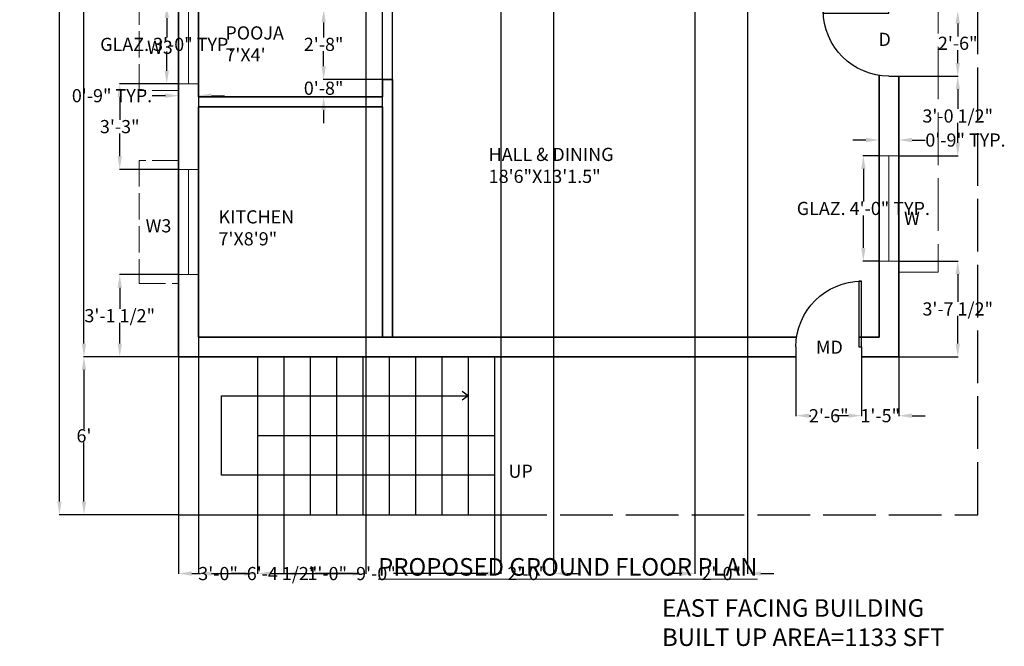
# Model space of a CAD drawing. Units: inches. Extents: x 515 to 964, y 435 to 999.
# Tile 1 of 2: x 515 to 964, y 435 to 721. Entities that reach past the tile are written whole.
import ezdxf

# ---------------------------------------------------------------- set-up
doc = ezdxf.new("R2010")
doc.units = ezdxf.units.IN
doc.header["$MEASUREMENT"] = 0
doc.linetypes.add('ACAD_ISO02W100', pattern=[15, 12, -3])
for name, color, linetype, lineweight in [('A-ANNO-DIMS', 2, 'Continuous', 18), ('A-ANNO-TEXT', 7, 'Continuous', 18), ('A-AREA-IDEN', 7, 'Continuous', 18), ('A-DOOR', 3, 'Continuous', 25), ('A-FLOR-OVHD', 8, 'ACAD_ISO02W100', 18), ('A-FLOR-STRS', 7, 'Continuous', 25), ('A-GLAZ', 4, 'Continuous', 18), ('A-WALL', 7, 'Continuous', 35), ('C-PROP', 8, 'ACAD_ISO02W100', 25)]:
    doc.layers.add(name, color=color, linetype=linetype, lineweight=lineweight)
doc.styles.get("Standard").update_dxf_attribs({"font": 'arial.ttf'})
doc.dimstyles.get("Standard").update_dxf_attribs({"dimtxt": 6, "dimasz": 6, "dimexe": 0.18, "dimexo": 0.0625, "dimgap": 0.09, "dimtad": 0, "dimtih": 1, "dimtoh": 1, "dimdec": 0, "dimzin": 0, "dimdsep": 46, "dimlunit": 3, "dimtxsty": 'Standard', "dimcen": 0.09, "dimadec": 0, "dimazin": 0, "dimtfac": 1, "dimtdec": 0, "dimtofl": 0, "dimtmove": 0, "dimatfit": 3, "dimfxl": 1, "dimtolj": 1, "dimtzin": 0, "dimarcsym": 0})

# ---------------------------------------------------------------- blocks, each defined once
blk = doc.blocks.new('*U2')
for p, q in [((0, 0), (0, -6)), ((40, 0), (40, -6))]:
    blk.add_line(p, q)
blk.add_lwpolyline([(0, 0), (0, 40), (1.75, 40), (1.75, 0)], close=True)
blk.add_arc((0, 0), 40, 0, 90)
blk = doc.blocks.new('*D5')
at = {"layer": 'A-ANNO-DIMS', "color": 0, "lineweight": -2, "transparency": 16777216}
for p, q in [((587.7, 945.51), (544.42, 945.51)), ((544.6, 939.51), (544.6, 759.42)), ((544.6, 573.01), (544.6, 753.11)), ((587.7, 567.01), (544.42, 567.01))]:
    blk.add_line(p, q, dxfattribs=at)
at = {"layer": 'A-ANNO-DIMS', "color": 0, "transparency": 16777216}
for points in [[(543.6, 939.51), (545.6, 939.51), (544.6, 945.51)], [(543.6, 573.01), (545.6, 573.01), (544.6, 567.01)]]:
    blk.add_solid(points, dxfattribs=at)
at = {"layer": 'Defpoints', "color": 0, "transparency": 16777216}
for p in [(587.76, 945.51), (544.6, 567.01), (587.76, 567.01)]:
    blk.add_point(p, dxfattribs=at)
at = {"layer": 'A-ANNO-DIMS', "color": 0, "transparency": 16777216, "insert": (544.6, 756.26), "char_height": 6, "attachment_point": 5}
blk.add_mtext('\\A1;31\'-7"', dxfattribs=at)
blk = doc.blocks.new('*D6')
at = {"layer": 'A-ANNO-DIMS', "color": 0, "lineweight": -2, "transparency": 16777216}
for p, q in [((587.7, 567.01), (544.42, 567.01)), ((544.6, 561.01), (544.6, 534.16)), ((544.6, 501.01), (544.6, 527.86)), ((587.7, 495.01), (544.42, 495.01))]:
    blk.add_line(p, q, dxfattribs=at)
at = {"layer": 'A-ANNO-DIMS', "color": 0, "transparency": 16777216}
for points in [[(543.6, 561.01), (545.6, 561.01), (544.6, 567.01)], [(543.6, 501.01), (545.6, 501.01), (544.6, 495.01)]]:
    blk.add_solid(points, dxfattribs=at)
at = {"layer": 'Defpoints', "color": 0, "transparency": 16777216}
for p in [(587.76, 567.01), (544.6, 495.01), (587.76, 495.01)]:
    blk.add_point(p, dxfattribs=at)
at = {"layer": 'A-ANNO-DIMS', "color": 0, "transparency": 16777216, "insert": (544.6, 531.01), "char_height": 6, "attachment_point": 5}
blk.add_mtext("\\A1;6'", dxfattribs=at)
blk = doc.blocks.new('GLAZ-48IN')
blk.add_line((4.5, 0), (4.5, 48))
blk.add_lwpolyline([(0, 0), (0, 48), (9, 48), (9, 0)], close=True)
blk = doc.blocks.new('GLAZ-36IN')
blk.add_line((0, 4.5), (36, 4.5))
blk.add_lwpolyline([(0, 9), (36, 9), (36, 0), (0, 0)], close=True)
blk = doc.blocks.new('*D10')
at = {"layer": 'A-ANNO-DIMS', "color": 0, "lineweight": -2, "transparency": 16777216}
for p, q in [((907.2, 658.68), (899.88, 658.68)), ((900.06, 652.68), (900.06, 637.87)), ((900.06, 616.68), (900.06, 631.49)), ((907.2, 610.68), (899.88, 610.68))]:
    blk.add_line(p, q, dxfattribs=at)
at = {"layer": 'A-ANNO-DIMS', "color": 0, "transparency": 16777216}
for points in [[(899.06, 652.68), (901.06, 652.68), (900.06, 658.68)], [(899.06, 616.68), (901.06, 616.68), (900.06, 610.68)]]:
    blk.add_solid(points, dxfattribs=at)
at = {"layer": 'Defpoints', "color": 0, "transparency": 16777216}
for p in [(900.06, 658.68), (907.26, 658.68), (907.26, 610.68)]:
    blk.add_point(p, dxfattribs=at)
at = {"layer": 'A-ANNO-DIMS', "color": 0, "transparency": 16777216, "insert": (900.06, 634.68), "char_height": 6, "attachment_point": 5}
blk.add_mtext('\\A1;GLAZ. 4\'-0" TYP.', dxfattribs=at)
blk = doc.blocks.new('*D11')
at = {"layer": 'A-ANNO-DIMS', "color": 0, "lineweight": -2, "transparency": 16777216}
for p, q in [((901.26, 665.88), (895.26, 665.88)), ((907.26, 658.74), (907.26, 666.06)), ((916.26, 658.74), (916.26, 666.06)), ((922.26, 665.88), (928.26, 665.88))]:
    blk.add_line(p, q, dxfattribs=at)
at = {"layer": 'A-ANNO-DIMS', "color": 0, "transparency": 16777216}
for points in [[(901.26, 666.88), (901.26, 664.88), (907.26, 665.88)], [(922.26, 666.88), (922.26, 664.88), (916.26, 665.88)]]:
    blk.add_solid(points, dxfattribs=at)
at = {"layer": 'Defpoints', "color": 0, "transparency": 16777216}
for p in [(916.26, 665.88), (907.26, 658.68), (916.26, 658.68)]:
    blk.add_point(p, dxfattribs=at)
at = {"layer": 'A-ANNO-DIMS', "color": 0, "transparency": 16777216, "insert": (946.64, 665.88), "char_height": 6, "attachment_point": 5}
blk.add_mtext('\\A1;0\'-9" TYP.', dxfattribs=at)
blk = doc.blocks.new('*D12')
at = {"layer": 'A-ANNO-DIMS', "color": 0, "lineweight": -2, "transparency": 16777216}
for p, q in [((587.7, 727.51), (582.18, 727.51)), ((582.36, 721.51), (582.36, 712.71)), ((582.36, 697.51), (582.36, 706.32)), ((587.7, 691.51), (582.18, 691.51))]:
    blk.add_line(p, q, dxfattribs=at)
at = {"layer": 'A-ANNO-DIMS', "color": 0, "transparency": 16777216}
for points in [[(581.36, 721.51), (583.36, 721.51), (582.36, 727.51)], [(581.36, 697.51), (583.36, 697.51), (582.36, 691.51)]]:
    blk.add_solid(points, dxfattribs=at)
at = {"layer": 'Defpoints', "color": 0, "transparency": 16777216}
for p in [(582.36, 727.51), (587.76, 727.51), (587.76, 691.51)]:
    blk.add_point(p, dxfattribs=at)
at = {"layer": 'A-ANNO-DIMS', "color": 0, "transparency": 16777216, "insert": (582.36, 709.51), "char_height": 6, "attachment_point": 5}
blk.add_mtext('\\A1;GLAZ. 3\'-0" TYP.', dxfattribs=at)
blk = doc.blocks.new('*D13')
at = {"layer": 'A-ANNO-DIMS', "color": 0, "lineweight": -2, "transparency": 16777216}
for p, q in [((587.76, 691.45), (587.76, 685.93)), ((596.76, 691.45), (596.76, 685.93)), ((581.76, 686.11), (575.76, 686.11)), ((602.76, 686.11), (608.76, 686.11))]:
    blk.add_line(p, q, dxfattribs=at)
at = {"layer": 'A-ANNO-DIMS', "color": 0, "transparency": 16777216}
for points in [[(581.76, 687.11), (581.76, 685.11), (587.76, 686.11)], [(602.76, 687.11), (602.76, 685.11), (596.76, 686.11)]]:
    blk.add_solid(points, dxfattribs=at)
at = {"layer": 'Defpoints', "color": 0, "transparency": 16777216}
for p in [(587.76, 691.51), (596.76, 691.51), (587.76, 686.11)]:
    blk.add_point(p, dxfattribs=at)
at = {"layer": 'A-ANNO-DIMS', "color": 0, "transparency": 16777216, "insert": (557.38, 686.11), "char_height": 6, "attachment_point": 5}
blk.add_mtext('\\A1;0\'-9" TYP.', dxfattribs=at)
blk = doc.blocks.new('*D17')
at = {"layer": 'A-ANNO-DIMS', "color": 0, "lineweight": -2, "transparency": 16777216}
for p, q in [((667.63, 963.51), (533.24, 963.51)), ((533.42, 957.51), (533.42, 732.46)), ((533.42, 501.01), (533.42, 726.07)), ((587.7, 495.01), (533.24, 495.01))]:
    blk.add_line(p, q, dxfattribs=at)
at = {"layer": 'A-ANNO-DIMS', "color": 0, "transparency": 16777216}
for points in [[(532.42, 957.51), (534.42, 957.51), (533.42, 963.51)], [(532.42, 501.01), (534.42, 501.01), (533.42, 495.01)]]:
    blk.add_solid(points, dxfattribs=at)
at = {"layer": 'Defpoints', "color": 0, "transparency": 16777216}
for p in [(533.42, 963.51), (667.69, 963.51), (587.76, 495.01)]:
    blk.add_point(p, dxfattribs=at)
at = {"layer": 'A-ANNO-DIMS', "color": 0, "transparency": 16777216, "insert": (533.42, 729.26), "char_height": 6, "attachment_point": 5}
blk.add_mtext('\\A1;39\'-0 1/2"', dxfattribs=at)
blk = doc.blocks.new('*D18')
at = {"layer": 'A-ANNO-DIMS', "color": 0, "lineweight": -2, "transparency": 16777216}
for p, q in [((623.76, 494.95), (623.76, 467.98)), ((731.76, 494.95), (731.76, 467.98)), ((629.76, 468.16), (669.7, 468.16)), ((725.76, 468.16), (685.83, 468.16))]:
    blk.add_line(p, q, dxfattribs=at)
at = {"layer": 'A-ANNO-DIMS', "color": 0, "transparency": 16777216}
for points in [[(629.76, 469.16), (629.76, 467.16), (623.76, 468.16)], [(725.76, 469.16), (725.76, 467.16), (731.76, 468.16)]]:
    blk.add_solid(points, dxfattribs=at)
at = {"layer": 'Defpoints', "color": 0, "transparency": 16777216}
for p in [(623.76, 495.01), (731.76, 495.01), (731.76, 468.16)]:
    blk.add_point(p, dxfattribs=at)
at = {"layer": 'A-ANNO-DIMS', "color": 0, "transparency": 16777216, "insert": (677.76, 468.16), "char_height": 6, "attachment_point": 5}
blk.add_mtext('\\A1;9\'-0"', dxfattribs=at)
blk = doc.blocks.new('*D19')
at = {"layer": 'A-ANNO-DIMS', "color": 0, "lineweight": -2, "transparency": 16777216}
for p, q in [((587.76, 494.95), (587.76, 467.98)), ((623.76, 494.95), (623.76, 467.98)), ((593.76, 468.16), (597.7, 468.16)), ((617.76, 468.16), (613.82, 468.16))]:
    blk.add_line(p, q, dxfattribs=at)
at = {"layer": 'A-ANNO-DIMS', "color": 0, "transparency": 16777216}
for points in [[(593.76, 469.16), (593.76, 467.16), (587.76, 468.16)], [(617.76, 469.16), (617.76, 467.16), (623.76, 468.16)]]:
    blk.add_solid(points, dxfattribs=at)
at = {"layer": 'Defpoints', "color": 0, "transparency": 16777216}
for p in [(587.76, 495.01), (623.76, 495.01), (623.76, 468.16)]:
    blk.add_point(p, dxfattribs=at)
at = {"layer": 'A-ANNO-DIMS', "color": 0, "transparency": 16777216, "insert": (605.76, 468.16), "char_height": 6, "attachment_point": 5}
blk.add_mtext('\\A1;3\'-0"', dxfattribs=at)
blk = doc.blocks.new('*D20')
at = {"layer": 'A-ANNO-DIMS', "color": 0, "lineweight": -2, "transparency": 16777216}
for p, q in [((623.76, 494.95), (623.76, 467.98)), ((635.76, 494.95), (635.76, 467.98)), ((617.76, 468.16), (611.76, 468.16)), ((641.76, 468.16), (647.76, 468.16))]:
    blk.add_line(p, q, dxfattribs=at)
at = {"layer": 'A-ANNO-DIMS', "color": 0, "transparency": 16777216}
for points in [[(617.76, 469.16), (617.76, 467.16), (623.76, 468.16)], [(641.76, 469.16), (641.76, 467.16), (635.76, 468.16)]]:
    blk.add_solid(points, dxfattribs=at)
at = {"layer": 'Defpoints', "color": 0, "transparency": 16777216}
for p in [(623.76, 495.01), (635.76, 495.01), (635.76, 468.16)]:
    blk.add_point(p, dxfattribs=at)
at = {"layer": 'A-ANNO-DIMS', "color": 0, "transparency": 16777216, "insert": (655.54, 468.16), "char_height": 6, "attachment_point": 5}
blk.add_mtext('\\A1;1\'-0"', dxfattribs=at)
blk = doc.blocks.new('*D21')
at = {"layer": 'A-ANNO-DIMS', "color": 0, "lineweight": -2, "transparency": 16777216}
for p, q in [((869.29, 566.95), (869.29, 539.98)), ((899.29, 566.95), (899.29, 539.98)), ((875.29, 540.16), (876.17, 540.16)), ((893.29, 540.16), (892.4, 540.16))]:
    blk.add_line(p, q, dxfattribs=at)
at = {"layer": 'A-ANNO-DIMS', "color": 0, "transparency": 16777216}
for points in [[(875.29, 541.16), (875.29, 539.16), (869.29, 540.16)], [(893.29, 541.16), (893.29, 539.16), (899.29, 540.16)]]:
    blk.add_solid(points, dxfattribs=at)
at = {"layer": 'Defpoints', "color": 0, "transparency": 16777216}
for p in [(869.29, 567.01), (899.29, 567.01), (869.29, 540.16)]:
    blk.add_point(p, dxfattribs=at)
at = {"layer": 'A-ANNO-DIMS', "color": 0, "transparency": 16777216, "insert": (884.29, 540.16), "char_height": 6, "attachment_point": 5}
blk.add_mtext('\\A1;2\'-6"', dxfattribs=at)
blk = doc.blocks.new('*D22')
at = {"layer": 'A-ANNO-DIMS', "color": 0, "lineweight": -2, "transparency": 16777216}
for p, q in [((899.29, 566.95), (899.29, 539.98)), ((916.26, 566.95), (916.26, 539.98)), ((893.29, 540.16), (887.29, 540.16)), ((922.26, 540.16), (928.26, 540.16))]:
    blk.add_line(p, q, dxfattribs=at)
at = {"layer": 'A-ANNO-DIMS', "color": 0, "transparency": 16777216}
for points in [[(893.29, 541.16), (893.29, 539.16), (899.29, 540.16)], [(922.26, 541.16), (922.26, 539.16), (916.26, 540.16)]]:
    blk.add_solid(points, dxfattribs=at)
at = {"layer": 'Defpoints', "color": 0, "transparency": 16777216}
for p in [(899.29, 567.01), (916.26, 567.01), (899.29, 540.16)]:
    blk.add_point(p, dxfattribs=at)
at = {"layer": 'A-ANNO-DIMS', "color": 0, "transparency": 16777216, "insert": (907.77, 540.16), "char_height": 6, "attachment_point": 5}
blk.add_mtext('\\A1;1\'-5"', dxfattribs=at)
blk = doc.blocks.new('*D23')
at = {"layer": 'A-ANNO-DIMS', "color": 0, "lineweight": -2, "transparency": 16777216}
for p, q in [((674.76, 990.36), (668.76, 990.36)), ((680.76, 576.07), (680.76, 990.54)), ((685.26, 576.07), (685.26, 990.54)), ((691.26, 990.36), (697.26, 990.36))]:
    blk.add_line(p, q, dxfattribs=at)
at = {"layer": 'A-ANNO-DIMS', "color": 0, "transparency": 16777216}
for points in [[(674.76, 991.36), (674.76, 989.36), (680.76, 990.36)], [(691.26, 991.36), (691.26, 989.36), (685.26, 990.36)]]:
    blk.add_solid(points, dxfattribs=at)
at = {"layer": 'Defpoints', "color": 0, "transparency": 16777216}
for p in [(685.26, 990.36), (680.76, 576.01), (685.26, 576.01)]:
    blk.add_point(p, dxfattribs=at)
at = {"layer": 'A-ANNO-DIMS', "color": 0, "transparency": 16777216, "insert": (712.32, 990.36), "char_height": 6, "attachment_point": 5}
blk.add_mtext('\\A1;0\'-4 1/2"', dxfattribs=at)
blk = doc.blocks.new('*D24')
at = {"layer": 'A-ANNO-DIMS', "color": 0, "lineweight": -2, "transparency": 16777216}
for p, q in [((596.76, 936.45), (596.76, 467.98)), ((673.1, 936.45), (673.1, 467.98)), ((602.76, 468.16), (619.86, 468.16)), ((667.1, 468.16), (650, 468.16))]:
    blk.add_line(p, q, dxfattribs=at)
at = {"layer": 'A-ANNO-DIMS', "color": 0, "transparency": 16777216}
for points in [[(602.76, 469.16), (602.76, 467.16), (596.76, 468.16)], [(667.1, 469.16), (667.1, 467.16), (673.1, 468.16)]]:
    blk.add_solid(points, dxfattribs=at)
at = {"layer": 'Defpoints', "color": 0, "transparency": 16777216}
for p in [(596.76, 936.51), (673.1, 936.51), (673.1, 468.16)]:
    blk.add_point(p, dxfattribs=at)
at = {"layer": 'A-ANNO-DIMS', "color": 0, "transparency": 16777216, "insert": (634.93, 468.16), "char_height": 6, "attachment_point": 5}
blk.add_mtext('\\A1;6\'-4 1/2"', dxfattribs=at)
blk = doc.blocks.new('*D25')
at = {"layer": 'A-ANNO-DIMS', "color": 0, "lineweight": -2, "transparency": 16777216}
for p, q in [((734.760949, 936.449016), (734.760949, 467.981516)), ((758.760949, 936.449016), (758.760949, 467.981516)), ((728.760949, 468.161516), (722.760949, 468.161516)), ((764.760949, 468.161516), (770.760949, 468.161516))]:
    blk.add_line(p, q, dxfattribs=at)
at = {"layer": 'A-ANNO-DIMS', "color": 0, "transparency": 16777216}
for points in [[(728.760949, 469.161516), (728.760949, 467.161516), (734.760949, 468.161516)], [(764.760949, 469.161516), (764.760949, 467.161516), (758.760949, 468.161516)]]:
    blk.add_solid(points, dxfattribs=at)
at = {"layer": 'Defpoints', "color": 0, "transparency": 16777216}
for p in [(734.760949, 936.511516), (758.760949, 936.511516), (758.760949, 468.161516)]:
    blk.add_point(p, dxfattribs=at)
at = {"layer": 'A-ANNO-DIMS', "color": 0, "transparency": 16777216, "insert": (746.760949, 468.161516), "char_height": 6, "attachment_point": 5}
blk.add_mtext('\\A1;2\'-0"', dxfattribs=at)
blk = doc.blocks.new('*D26')
at = {"layer": 'A-ANNO-DIMS', "color": 0, "lineweight": -2, "transparency": 16777216}
for p, q in [((823.260949, 936.449016), (823.260949, 467.981516)), ((847.260949, 936.449016), (847.260949, 467.981516)), ((817.260949, 468.161516), (811.260949, 468.161516)), ((853.260949, 468.161516), (859.260949, 468.161516))]:
    blk.add_line(p, q, dxfattribs=at)
at = {"layer": 'A-ANNO-DIMS', "color": 0, "transparency": 16777216}
for points in [[(817.260949, 469.161516), (817.260949, 467.161516), (823.260949, 468.161516)], [(853.260949, 469.161516), (853.260949, 467.161516), (847.260949, 468.161516)]]:
    blk.add_solid(points, dxfattribs=at)
at = {"layer": 'Defpoints', "color": 0, "transparency": 16777216}
for p in [(823.260949, 936.511516), (847.260949, 936.511516), (847.260949, 468.161516)]:
    blk.add_point(p, dxfattribs=at)
at = {"layer": 'A-ANNO-DIMS', "color": 0, "transparency": 16777216, "insert": (835.260949, 468.161516), "char_height": 6, "attachment_point": 5}
blk.add_mtext('\\A1;2\'-0"', dxfattribs=at)
blk = doc.blocks.new('*D27')
at = {"layer": 'A-ANNO-DIMS', "color": 0, "lineweight": -2, "transparency": 16777216}
for p, q in [((587.7, 604.51), (560.73, 604.51)), ((560.91, 598.51), (560.91, 588.96)), ((560.91, 573.01), (560.91, 582.57)), ((587.7, 567.01), (560.73, 567.01))]:
    blk.add_line(p, q, dxfattribs=at)
at = {"layer": 'A-ANNO-DIMS', "color": 0, "transparency": 16777216}
for points in [[(559.91, 598.51), (561.91, 598.51), (560.91, 604.51)], [(559.91, 573.01), (561.91, 573.01), (560.91, 567.01)]]:
    blk.add_solid(points, dxfattribs=at)
at = {"layer": 'Defpoints', "color": 0, "transparency": 16777216}
for p in [(560.91, 604.51), (587.76, 604.51), (587.76, 567.01)]:
    blk.add_point(p, dxfattribs=at)
at = {"layer": 'A-ANNO-DIMS', "color": 0, "transparency": 16777216, "insert": (560.91, 585.76), "char_height": 6, "attachment_point": 5}
blk.add_mtext('\\A1;3\'-1 1/2"', dxfattribs=at)
blk = doc.blocks.new('*D28')
at = {"layer": 'A-ANNO-DIMS', "color": 0, "lineweight": -2, "transparency": 16777216}
for p, q in [((587.7, 691.51), (560.73, 691.51)), ((560.91, 685.51), (560.91, 675.17)), ((560.91, 658.51), (560.91, 668.86)), ((587.7, 652.51), (560.73, 652.51))]:
    blk.add_line(p, q, dxfattribs=at)
at = {"layer": 'A-ANNO-DIMS', "color": 0, "transparency": 16777216}
for points in [[(559.91, 685.51), (561.91, 685.51), (560.91, 691.51)], [(559.91, 658.51), (561.91, 658.51), (560.91, 652.51)]]:
    blk.add_solid(points, dxfattribs=at)
at = {"layer": 'Defpoints', "color": 0, "transparency": 16777216}
for p in [(560.91, 691.51), (587.76, 691.51), (587.76, 652.51)]:
    blk.add_point(p, dxfattribs=at)
at = {"layer": 'A-ANNO-DIMS', "color": 0, "transparency": 16777216, "insert": (560.91, 672.01), "char_height": 6, "attachment_point": 5}
blk.add_mtext('\\A1;3\'-3"', dxfattribs=at)
blk = doc.blocks.new('*D30')
at = {"layer": 'A-ANNO-DIMS', "color": 0, "lineweight": -2, "transparency": 16777216}
for p, q in [((916.32, 610.68), (943.29, 610.68)), ((943.11, 604.68), (943.11, 592.04)), ((943.11, 573.01), (943.11, 585.65)), ((916.32, 567.01), (943.29, 567.01))]:
    blk.add_line(p, q, dxfattribs=at)
at = {"layer": 'A-ANNO-DIMS', "color": 0, "transparency": 16777216}
for points in [[(942.11, 604.68), (944.11, 604.68), (943.11, 610.68)], [(942.11, 573.01), (944.11, 573.01), (943.11, 567.01)]]:
    blk.add_solid(points, dxfattribs=at)
at = {"layer": 'Defpoints', "color": 0, "transparency": 16777216}
for p in [(916.26, 610.68), (916.26, 567.01), (943.11, 567.01)]:
    blk.add_point(p, dxfattribs=at)
at = {"layer": 'A-ANNO-DIMS', "color": 0, "transparency": 16777216, "insert": (943.11, 588.85), "char_height": 6, "attachment_point": 5}
blk.add_mtext('\\A1;3\'-7 1/2"', dxfattribs=at)
blk = doc.blocks.new('*D31')
at = {"layer": 'A-ANNO-DIMS', "color": 0, "lineweight": -2, "transparency": 16777216}
for p, q in [((916.32, 695.01), (943.29, 695.01)), ((943.11, 689.01), (943.11, 680.04)), ((943.11, 664.68), (943.11, 673.65)), ((916.32, 658.68), (943.29, 658.68))]:
    blk.add_line(p, q, dxfattribs=at)
at = {"layer": 'A-ANNO-DIMS', "color": 0, "transparency": 16777216}
for points in [[(942.11, 689.01), (944.11, 689.01), (943.11, 695.01)], [(942.11, 664.68), (944.11, 664.68), (943.11, 658.68)]]:
    blk.add_solid(points, dxfattribs=at)
at = {"layer": 'Defpoints', "color": 0, "transparency": 16777216}
for p in [(916.26, 695.01), (916.26, 658.68), (943.11, 658.68)]:
    blk.add_point(p, dxfattribs=at)
at = {"layer": 'A-ANNO-DIMS', "color": 0, "transparency": 16777216, "insert": (943.11, 676.85), "char_height": 6, "attachment_point": 5}
blk.add_mtext('\\A1;3\'-0 1/2"', dxfattribs=at)
blk = doc.blocks.new('*D32')
at = {"layer": 'A-ANNO-DIMS', "color": 0, "lineweight": -2, "transparency": 16777216}
for p, q in [((916.32, 725.01), (943.29, 725.01)), ((943.11, 719.01), (943.11, 713.16)), ((943.11, 701.01), (943.11, 706.86)), ((916.32, 695.01), (943.29, 695.01))]:
    blk.add_line(p, q, dxfattribs=at)
at = {"layer": 'A-ANNO-DIMS', "color": 0, "transparency": 16777216}
for points in [[(942.11, 719.01), (944.11, 719.01), (943.11, 725.01)], [(942.11, 701.01), (944.11, 701.01), (943.11, 695.01)]]:
    blk.add_solid(points, dxfattribs=at)
at = {"layer": 'Defpoints', "color": 0, "transparency": 16777216}
for p in [(916.26, 725.01), (916.26, 695.01), (943.11, 695.01)]:
    blk.add_point(p, dxfattribs=at)
at = {"layer": 'A-ANNO-DIMS', "color": 0, "transparency": 16777216, "insert": (943.11, 710.01), "char_height": 6, "attachment_point": 5}
blk.add_mtext('\\A1;2\'-6"', dxfattribs=at)
blk = doc.blocks.new('*D34')
at = {"layer": 'A-ANNO-DIMS', "color": 0, "lineweight": -2, "transparency": 16777216}
for p, q in [((680.7, 725.51), (653.73, 725.51)), ((653.91, 719.51), (653.91, 712.66)), ((653.91, 699.51), (653.91, 706.36)), ((680.7, 693.51), (653.73, 693.51))]:
    blk.add_line(p, q, dxfattribs=at)
at = {"layer": 'A-ANNO-DIMS', "color": 0, "transparency": 16777216}
for points in [[(652.91, 719.51), (654.91, 719.51), (653.91, 725.51)], [(652.91, 699.51), (654.91, 699.51), (653.91, 693.51)]]:
    blk.add_solid(points, dxfattribs=at)
at = {"layer": 'Defpoints', "color": 0, "transparency": 16777216}
for p in [(653.91, 725.51), (680.76, 725.51), (680.76, 693.51)]:
    blk.add_point(p, dxfattribs=at)
at = {"layer": 'A-ANNO-DIMS', "color": 0, "transparency": 16777216, "insert": (653.91, 709.51), "char_height": 6, "attachment_point": 5}
blk.add_mtext('\\A1;2\'-8"', dxfattribs=at)
blk = doc.blocks.new('*D35')
at = {"layer": 'A-ANNO-DIMS', "color": 0, "lineweight": -2, "transparency": 16777216}
for p, q in [((653.910949, 699.511516), (653.910949, 705.511516)), ((680.698449, 693.511516), (653.730949, 693.511516)), ((680.698449, 685.511516), (653.730949, 685.511516)), ((653.910949, 679.511516), (653.910949, 673.511516))]:
    blk.add_line(p, q, dxfattribs=at)
at = {"layer": 'A-ANNO-DIMS', "color": 0, "transparency": 16777216}
for points in [[(652.910949, 699.511516), (654.910949, 699.511516), (653.910949, 693.511516)], [(652.910949, 679.511516), (654.910949, 679.511516), (653.910949, 685.511516)]]:
    blk.add_solid(points, dxfattribs=at)
at = {"layer": 'Defpoints', "color": 0, "transparency": 16777216}
for p in [(653.910949, 693.511516), (680.760949, 693.511516), (680.760949, 685.511516)]:
    blk.add_point(p, dxfattribs=at)
at = {"layer": 'A-ANNO-DIMS', "color": 0, "transparency": 16777216, "insert": (653.910949, 689.511516), "char_height": 6, "attachment_point": 5}
blk.add_mtext('\\A1;0\'-8"', dxfattribs=at)

msp = doc.modelspace()

# ---------------------------------------------------------------- linework, layer by layer
at = {"layer": 'A-FLOR-OVHD'}
for p, q in [((587.76, 656.62), (569.76, 656.62)), ((569.76, 656.62), (569.76, 600.39)), ((569.76, 600.39), (587.76, 600.39))]:
    msp.add_line(p, q, dxfattribs=at)
at = {"layer": 'A-FLOR-OVHD', "ltscale": 2}
msp.add_lwpolyline([(916.26, 828.46), (934.26, 828.46), (934.26, 605.63), (916.26, 605.63)], dxfattribs=at)
at = {"layer": 'A-FLOR-OVHD'}
msp.add_lwpolyline([(587.76, 688.47), (569.76, 688.47), (569.76, 731.11)], dxfattribs=at)
at = {"layer": 'A-FLOR-STRS'}
for p, q in [((587.76, 567.01), (587.76, 495.01)), ((623.76, 567.01), (623.76, 495.01)), ((635.76, 567.01), (635.76, 495.01)), ((647.76, 567.01), (647.76, 495.01)), ((659.76, 567.01), (659.76, 495.01)), ((671.76, 567.01), (671.76, 495.01)), ((683.76, 567.01), (683.76, 495.01)), ((695.76, 567.01), (695.76, 495.01)), ((707.76, 567.01), (707.76, 495.01)), ((719.76, 567.01), (719.76, 495.01)), ((731.76, 567.01), (731.76, 495.01)), ((607.31, 513.01), (607.31, 549.22)), ((607.31, 549.22), (719.76, 549.22)), ((719.76, 549.22), (717.09, 551.23)), ((719.76, 549.22), (717.09, 547.2)), ((731.76, 531.01), (623.76, 531.01)), ((731.76, 513.01), (607.31, 513.01)), ((587.76, 495.01), (731.76, 495.01))]:
    msp.add_line(p, q, dxfattribs=at)
at = {"layer": 'A-WALL'}
for p, q in [((596.76, 685.51), (596.76, 733.51)), ((680.76, 685.51), (680.76, 693.51)), ((680.76, 693.51), (685.26, 693.51)), ((685.26, 576.01), (685.26, 693.51)), ((907.26, 695.35), (907.26, 576.01)), ((680.76, 685.51), (596.76, 685.51)), ((596.76, 576.01), (596.76, 681.01)), ((680.76, 681.01), (596.76, 681.01)), ((680.76, 576.01), (680.76, 681.01)), ((869.63, 576.01), (596.76, 576.01)), ((907.26, 576.01), (897.98, 576.01))]:
    msp.add_line(p, q, dxfattribs=at)
for points in [[(869.29, 567.01), (587.76, 567.01), (587.76, 945.51), (916.26, 945.51), (916.26, 725.01)], [(916.26, 695.01), (916.26, 567.01), (899.29, 567.01)]]:
    msp.add_lwpolyline(points, dxfattribs=at)
at = {"layer": 'C-PROP', "ltscale": 2}
for p, q in [((952.26, 495.01), (952.26, 945.51)), ((731.76, 495.01), (952.26, 495.01))]:
    msp.add_line(p, q, dxfattribs=at)

# ---------------------------------------------------------------- block references
at = {"layer": 'A-DOOR', "xscale": -0.75, "yscale": 0.75, "zscale": 0.75}
for p, rotation in [((911.76, 725.01), 90), ((899.29, 571.51), 359.9999999999999)]:
    msp.add_blockref('*U2', p, dxfattribs=dict(at, rotation=rotation))
at = {"layer": 'A-GLAZ', "rotation": 90}
msp.add_blockref('GLAZ-36IN', (596.76, 691.51), dxfattribs=at)
at = {"layer": 'A-GLAZ'}
for p in [(907.26, 610.68), (587.76, 604.51)]:
    msp.add_blockref('GLAZ-48IN', p, dxfattribs=at)

# ---------------------------------------------------------------- texts
at = {"layer": 'A-ANNO-TEXT', "attachment_point": 1}
for s, width, insert, char_height in [('D', 31.2334, (906.97, 714.78), 6), ('W3', 46.9696, (573.35, 711.19), 6), ('W3', 46.9696, (572.72, 629.76), 6), ('W', 46.9696, (918.62, 633.17), 6), ('MD', 31.2334, (878.43, 574.41), 6), ('UP', 44.1471, (738.19, 517.83), 6), ('{\\fArial|b1|i0|c0|p34;\\LPROPOSED GROUND FLOOR PLAN}', 234.7669, (678.77, 475.21), 8), ('{\\fArial|b1|i0|c0|p34;EAST FACING BUILDING\\PBUILT UP AREA=1133 SFT}', 379.9738, (808.26, 456.46), 8)]:
    msp.add_mtext_dynamic_manual_height_columns(s, width=width, gutter_width=1, heights=[0], dxfattribs=dict(at, insert=insert, char_height=char_height))
at = {"layer": 'A-AREA-IDEN', "char_height": 6, "attachment_point": 1}
for s, insert in [("POOJA\\P7'X4'", (609.1, 717.73)), ('HALL & DINING \\P18\'6"X13\'1.5"', (729.17, 662.32)), ('KITCHEN\\P7\'X8\'9"', (605.96, 633.83))]:
    msp.add_mtext_dynamic_manual_height_columns(s, width=150.2085, gutter_width=1, heights=[0], dxfattribs=dict(at, insert=insert))

# ---------------------------------------------------------------- dimensions: what is measured, and where the dimension line sits
at = {"layer": 'A-ANNO-DIMS'}
for base, p1, p2, picture, middle in [((685.26, 990.36), (680.76, 576.01), (685.26, 576.01), '*D23', (712.32, 990.36)), ((673.1, 468.16), (596.76, 936.51), (673.1, 936.51), '*D24', (634.93, 468.16)), ((758.76, 468.16), (734.76, 936.51), (758.76, 936.51), '*D25', (746.76, 468.16)), ((847.26, 468.16), (823.26, 936.51), (847.26, 936.51), '*D26', (835.26, 468.16)), ((623.76, 468.16), (587.76, 495.01), (623.76, 495.01), '*D19', (605.76, 468.16)), ((635.76, 468.16), (623.76, 495.01), (635.76, 495.01), '*D20', (655.54, 468.16)), ((731.76, 468.16), (623.76, 495.01), (731.76, 495.01), '*D18', (677.76, 468.16))]:
    dim = msp.add_linear_dim(base=base, p1=p1, p2=p2, dimstyle='Standard', override={"dimdec": 1, "dimlfac": 1, "dimrnd": 0, "dimzin": 1, "dimdsep": 46, "dimlunit": 4, "dimfrac": 2}, dxfattribs=at)
    dim.commit()
    dim.dimension.update_dxf_attribs({"geometry": picture, "text_midpoint": middle})
for base, p1, p2, angle, override, picture, middle in [((533.42, 963.51), (587.76, 495.01), (667.69, 963.51), 90, {"dimdec": 1, "dimlfac": 1, "dimrnd": 0, "dimzin": 1, "dimdsep": 46, "dimlunit": 4, "dimfrac": 2}, '*D17', (533.42, 729.26)), ((544.59562099, 567.01151569), (587.76094904, 945.51151569), (587.76094904, 567.01151569), 90, {"dimclrd": 0, "dimclre": 0, "dimclrt": 0}, '*D5', (544.59562099, 756.26151569)), ((653.91, 725.51), (680.76, 693.51), (680.76, 725.51), 90, {"dimdec": 1, "dimlfac": 1, "dimrnd": 0, "dimzin": 1, "dimdsep": 46, "dimlunit": 4, "dimfrac": 2}, '*D34', (653.91, 709.51)), ((943.11, 695.01), (916.26, 725.01), (916.26, 695.01), 270, {"dimdec": 1, "dimlfac": 1, "dimrnd": 0, "dimzin": 1, "dimdsep": 46, "dimlunit": 4, "dimfrac": 2}, '*D32', (943.11, 710.01)), ((653.91, 693.51), (680.76, 685.51), (680.76, 693.51), 90, {"dimdec": 1, "dimlfac": 1, "dimrnd": 0, "dimzin": 1, "dimdsep": 46, "dimlunit": 4, "dimfrac": 2}, '*D35', (653.91, 689.51)), ((943.11, 658.68), (916.26, 695.01), (916.26, 658.68), 270, {"dimdec": 1, "dimlfac": 1, "dimrnd": 0, "dimzin": 1, "dimdsep": 46, "dimlunit": 4, "dimfrac": 2}, '*D31', (943.11, 676.85)), ((560.91, 691.51), (587.76, 652.51), (587.76, 691.51), 90, {"dimdec": 1, "dimlfac": 1, "dimrnd": 0, "dimzin": 1, "dimdsep": 46, "dimlunit": 4, "dimfrac": 2}, '*D28', (560.91, 672.01)), ((943.11, 567.01), (916.26, 610.68), (916.26, 567.01), 270, {"dimdec": 1, "dimlfac": 1, "dimrnd": 0, "dimzin": 1, "dimdsep": 46, "dimlunit": 4, "dimfrac": 2}, '*D30', (943.11, 588.85)), ((560.91, 604.51), (587.76, 567.01), (587.76, 604.51), 90, {"dimdec": 1, "dimlfac": 1, "dimrnd": 0, "dimzin": 1, "dimdsep": 46, "dimlunit": 4, "dimfrac": 2}, '*D27', (560.91, 585.76)), ((544.6, 495.01), (587.76, 567.01), (587.76, 495.01), 90, {"dimclrd": 0, "dimclre": 0, "dimclrt": 0, "dimtmove": 1}, '*D6', (544.6, 531.01)), ((869.29, 540.16), (899.29, 567.01), (869.29, 567.01), 180, {"dimdec": 1, "dimlfac": 1, "dimrnd": 0, "dimzin": 1, "dimdsep": 46, "dimlunit": 4, "dimfrac": 2}, '*D21', (884.29, 540.16)), ((899.29, 540.16), (916.26, 567.01), (899.29, 567.01), 180, {"dimdec": 1, "dimlfac": 1, "dimrnd": 0, "dimzin": 1, "dimdsep": 46, "dimlunit": 4, "dimfrac": 2}, '*D22', (907.77, 540.16))]:
    dim = msp.add_linear_dim(base=base, p1=p1, p2=p2, angle=angle, dimstyle='Standard', override=override, dxfattribs=at)
    dim.commit()
    dim.dimension.update_dxf_attribs({"geometry": picture, "text_midpoint": middle})
for base, p1, p2, angle, text, picture, middle in [((582.36, 727.51), (587.76, 691.51), (587.76, 727.51), 90, 'GLAZ. <> TYP.', '*D12', (582.36, 709.51)), ((587.76, 686.11), (596.76, 691.51), (587.76, 691.51), 180, '<> TYP.', '*D13', (557.38, 686.11)), ((900.06, 658.68), (907.26, 610.68), (907.26, 658.68), 90, 'GLAZ. <> TYP.', '*D10', (900.06, 634.68))]:
    dim = msp.add_linear_dim(base=base, p1=p1, p2=p2, angle=angle, text=text, dimstyle='Standard', override={"dimdec": 1, "dimlfac": 1, "dimrnd": 0, "dimzin": 1, "dimdsep": 46, "dimlunit": 4, "dimfrac": 2}, dxfattribs=at)
    dim.commit()
    dim.dimension.update_dxf_attribs({"geometry": picture, "text_midpoint": middle})
dim = msp.add_linear_dim(base=(916.26, 665.88), p1=(907.26, 658.68), p2=(916.26, 658.68), text='<> TYP.', dimstyle='Standard', override={"dimdec": 1, "dimlfac": 1, "dimrnd": 0, "dimzin": 1, "dimdsep": 46, "dimlunit": 4, "dimfrac": 2}, dxfattribs=at)
dim.commit()
dim.dimension.update_dxf_attribs({"geometry": '*D11', "text_midpoint": (946.64, 665.88)})

doc.saveas('drawing.dxf')
